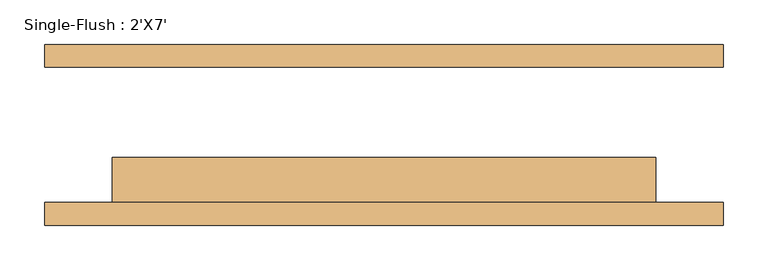
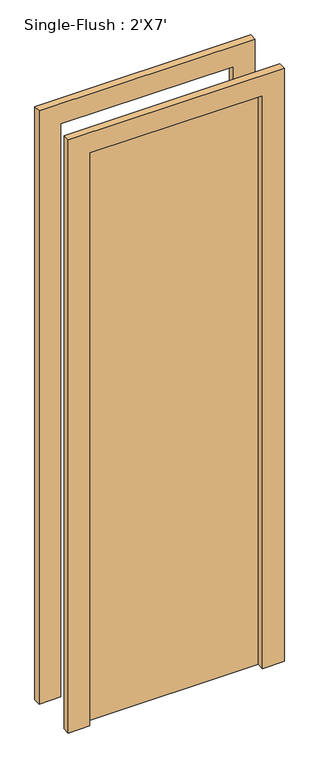
"""IFC4 building model written with IfcOpenShell, lengths in millimetres: door geometry, Single-Flush : 2'X7'."""

from ifc_helpers import new_model, si_unit, frame, origin, origin_with_axes, place, context, project, spatial, polyline, outline, extrude, source, transform, mapped, element, save


def single_flush_2_x7_5ca4d175(model_context):
    return source(origin(), model_context, "Body", "SweptSolid", [
        extrude(outline(polyline([(2209.8, -381.0), (0.0, -381.0), (0.0, -304.8), (2133.6, -304.8), (2133.6, 304.8), (0.0, 304.8), (0.0, 381.0), (2209.8, 381.0), (2209.8, -381.0)])), frame((0.0, -101.6, 0.0), z_axis=(0.0, 1.0, 0.0), x_axis=(0.0, 0.0, 1.0)), (0.0, 0.0, 1.0), 25.4),
        extrude(outline(polyline([(2209.8, 381.0), (2209.8, -381.0), (0.0, -381.0), (0.0, -304.8), (2133.6, -304.8), (2133.6, 304.8), (0.0, 304.8), (0.0, 381.0), (2209.8, 381.0)])), frame((0.0, 76.2, 0.0), z_axis=(0.0, 1.0, 0.0), x_axis=(0.0, 0.0, 1.0)), (0.0, 0.0, 1.0), 25.4),
        extrude(outline(polyline([(304.8, -25.4), (304.8, -76.2), (-304.8, -76.2), (-304.8, -25.4), (304.8, -25.4)])), origin_with_axes(), (0.0, 0.0, 1.0), 2133.6),
    ])


if __name__ == "__main__":
    model = new_model("IFC4")
    model_context = context("Model", 3, world=origin())
    ifc_project = project(units=[si_unit("LENGTHUNIT", "METRE", prefix="MILLI")], contexts=[model_context])
    site = spatial("IfcSite", under=ifc_project)
    building = spatial("IfcBuilding", under=site)
    placement = place(None, origin())
    single_flush_2_x7_shape = single_flush_2_x7_5ca4d175(model_context)
    element("IfcDoor", 1, ObjectType="Single-Flush : 2'X7'", at=placement, inside=building, context=model_context, shape_type="MappedRepresentation", body=[
        mapped(single_flush_2_x7_shape, transform((0.0, 0.0, 0.0), x_axis=(1.0, 0.0, 0.0), y_axis=(0.0, 1.0, 0.0), z_axis=(0.0, 0.0, 1.0))),
    ])
    save(model, "model.ifc")

# Revit data of these elements
# Type "Single-Flush : 2'X7'"
#   Type Mark = "12"
#   Construction Type Id = "MDOOR"
#   Assembly Code = "C1020"
#   Analytic Construction = "Metal"
#   Thickness = 0' - 2"
#   Heat Transfer Coefficient (U) = 0.651978 BTU/(h·ft²·°F)
#   Height = 7' - 0"
#   Trim Projection Ext = 0' - 1"
#   Trim Projection Int = 0' - 1"
#   Trim Width = 0' - 3"
#   Width = 2' - 0"
#   Define Thermal Properties by = 1
#   Door Material = Door - Panel
#   Frame Material = Door - Frame
#   Visual Light Transmittance = 0
#   Solar Heat Gain Coefficient = 0
#   Function = (empty or 0)
#   Wall Closure = (empty or 0)
# Element 1 (IfcDoor, "Single-Flush : 2'X7'")
#   Materials on its faces: "Door - Frame", "Door - Panel"
# Materials
#   "Door - Panel": class "Wood", colour RGB 210 159 95, transparency 0, Cost = 0
#   "Door - Frame": colour RGB 118 70 51, transparency 0, Cost = 0
